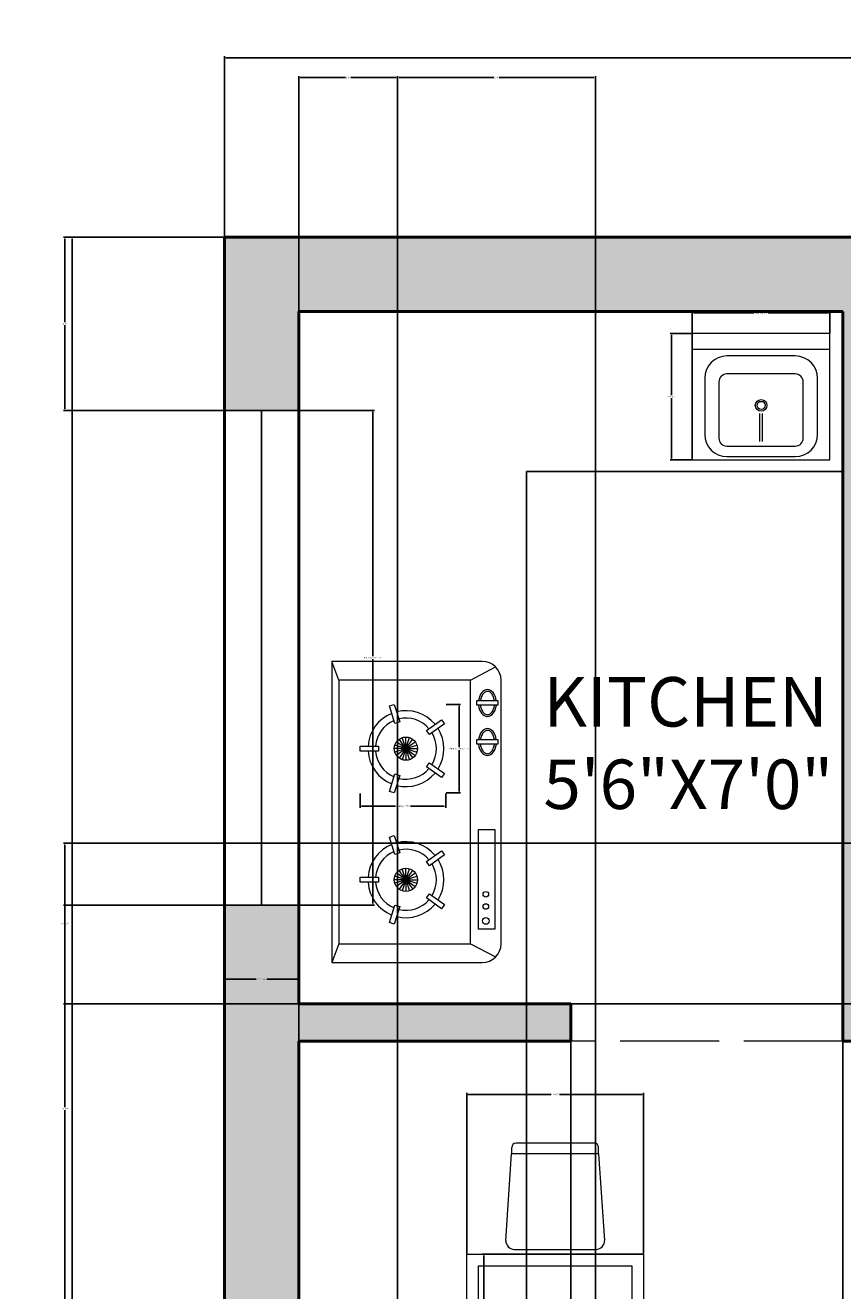
# Model space of a CAD drawing. Units: inches. Extents: x -2 to 282, y -370 to 35.
# Tile 4 of 5: x -2 to 97, y -119 to 35. Entities that reach past the tile are written whole.
import ezdxf

# ---------------------------------------------------------------- set-up
doc = ezdxf.new("R2010")
doc.units = ezdxf.units.IN
doc.header["$MEASUREMENT"] = 0
doc.linetypes.add('ACAD_ISO02W100', pattern=[15, 12, -3])
for name, color, linetype, lineweight in [('A-ANNO-DIMS', 2, 'Continuous', 18), ('A-AREA-IDEN', 7, 'Continuous', 25), ('A-EQPM', 8, 'Continuous', 18), ('A-FLOR-CASE', 8, 'Continuous', 25), ('A-FLOR-FIXT', 9, 'Continuous', 18), ('A-FURN', 8, 'Continuous', 18), ('A-GLAZ', 4, 'Continuous', 25), ('A-WALL', 7, 'Continuous', 50), ('A-WALL-OVHD', 7, 'ACAD_ISO02W100', 18), ('A-WALL-PATT', 252, 'Continuous', 13)]:
    doc.layers.add(name, color=color, linetype=linetype, lineweight=lineweight)
doc.styles.get("Standard").update_dxf_attribs({"font": 'arial.ttf'})
doc.dimstyles.get("Standard").update_dxf_attribs({"dimtxt": 0.18, "dimasz": 0.18, "dimexe": 0.18, "dimexo": 0.0625, "dimgap": 0.09, "dimtad": 0, "dimtih": 1, "dimtoh": 1, "dimdec": 0, "dimzin": 0, "dimdsep": 46, "dimlunit": 3, "dimtxsty": 'Standard', "dimcen": 0.09, "dimadec": 0, "dimazin": 0, "dimtfac": 1, "dimtdec": 0, "dimtofl": 0, "dimtmove": 0, "dimatfit": 3, "dimfxl": 1, "dimtolj": 1, "dimtzin": 0, "dimarcsym": 0})

# ---------------------------------------------------------------- blocks, each defined once
blk = doc.blocks.new('*D2')
at = {"layer": 'A-ANNO-DIMS', "color": 0, "lineweight": -2, "transparency": 16777216}
for p, q in [((22.35, 9.19), (3.74, 9.19)), ((3.92, 9.01), (3.92, -167.65)), ((3.92, -350.63), (3.92, -173.97)), ((22.35, -350.81), (3.74, -350.81))]:
    blk.add_line(p, q, dxfattribs=at)
at = {"layer": 'A-ANNO-DIMS', "color": 0, "transparency": 16777216}
for points in [[(3.89, 9.01), (3.95, 9.01), (3.92, 9.19)], [(3.89, -350.63), (3.95, -350.63), (3.92, -350.81)]]:
    blk.add_solid(points, dxfattribs=at)
at = {"layer": 'Defpoints', "color": 0, "transparency": 16777216}
for p in [(3.92, 9.19), (22.41, 9.19), (22.41, -350.81)]:
    blk.add_point(p, dxfattribs=at)
at = {"layer": 'A-ANNO-DIMS', "color": 0, "transparency": 16777216, "insert": (3.92, -170.81), "char_height": 6, "attachment_point": 5}
blk.add_mtext("\\A1;30'", dxfattribs=at)
blk = doc.blocks.new('*D3')
at = {"layer": 'A-ANNO-DIMS', "color": 0, "lineweight": -2, "transparency": 16777216}
for p, q in [((22.41, 9.25), (22.41, 31.14)), ((22.59, 30.96), (137.18, 30.96)), ((262.23, 30.96), (147.65, 30.96)), ((262.41, 9.25), (262.41, 31.14))]:
    blk.add_line(p, q, dxfattribs=at)
at = {"layer": 'A-ANNO-DIMS', "color": 0, "transparency": 16777216}
for points in [[(22.59, 30.99), (22.59, 30.93), (22.41, 30.96)], [(262.23, 30.99), (262.23, 30.93), (262.41, 30.96)]]:
    blk.add_solid(points, dxfattribs=at)
at = {"layer": 'Defpoints', "color": 0, "transparency": 16777216}
for p in [(262.41, 30.96), (22.41, 9.19), (262.41, 9.19)]:
    blk.add_point(p, dxfattribs=at)
at = {"layer": 'A-ANNO-DIMS', "color": 0, "transparency": 16777216, "insert": (142.41, 30.96), "char_height": 6, "attachment_point": 5}
blk.add_mtext("\\A1;20'", dxfattribs=at)
blk = doc.blocks.new('М14 600х655')
for p, q in [((-655, 600), (-655, 0)), ((-655, 600), (-655, 0)), ((-655, 0), (-655, 600)), ((0, 600), (-655, 600)), ((0, 0), (0, 600)), ((0, 525), (-655, 525)), ((-165.1, 494.1), (-489.9, 494.1)), ((-595.8, 388.1), (-595.8, 121.3)), ((-528.4, 370.1), (-528.4, 103.3)), ((-165.4, 408.4), (-490.2, 408.4)), ((-127.2, 103.3), (-127.2, 370.1)), ((-59.2, 121.3), (-59.2, 388.1)), ((-333.5, 87.1), (-333.5, 219.6)), ((-321.5, 87.1), (-321.5, 219.6)), ((-490.2, 65.1), (-165.4, 65.1)), ((-655, 0), (-655, 0)), ((-655, 0), (-655, 0)), ((-655, 0), (0, 0)), ((-655, 0), (0, 0)), ((-489.9, 15.4), (-165.1, 15.4))]:
    blk.add_line(p, q)
for radius in [27.6, 19.3]:
    blk.add_circle((-327.5, 258.9), radius)
for centre, radius, start, end in [((-489.9, 388.1), 105.9, 90, 180), ((-165.1, 388.1), 105.9, 0, 90), ((-490.2, 370.1), 38.2, 90, 180), ((-165.4, 370.1), 38.2, 0, 90), ((-489.9, 121.3), 105.9, 180, 270), ((-165.1, 121.3), 105.9, 270, 0), ((-490.2, 103.3), 38.2, 180, 270), ((-165.4, 103.3), 38.2, 270, 0)]:
    blk.add_arc(centre, radius, start, end)
blk = doc.blocks.new('WINDOW-60IN')
for p, q in [((0, 0), (0, 60)), ((0, 60), (9, 60)), ((4.5, 60), (4.5, 0)), ((9, 60), (9, 0)), ((9, 0), (0, 0))]:
    blk.add_line(p, q)
blk = doc.blocks.new('DINING-CHAIR')
for p, q in [((0.71, 12.36), (0.71, 11.58)), ((10.75, 12.87), (1.23, 12.87)), ((11.26, 11.58), (11.26, 12.36)), ((0, 1.09), (0.71, 11.58)), ((11.26, 11.58), (0.71, 11.58)), ((11.26, 11.58), (11.98, 1.09)), ((1.03, 0), (10.95, 0))]:
    blk.add_line(p, q)
for centre, radius, start, end in [((1.23, 12.36), 0.515, 90, 180), ((10.75, 12.36), 0.515, 0, 90), ((1.03, 1.03), 1.03, 176.8779, 270), ((10.95, 1.03), 1.03, 270, 3.1221)]:
    blk.add_arc(centre, radius, start, end)
blk = doc.blocks.new('COOKTOP-BURNER')
for p, q in [((3.54, 10.55), (4.13, 10.74)), ((4.22, 8.44), (3.54, 10.55)), ((4.13, 10.74), (4.82, 8.63)), ((4.82, 8.63), (4.22, 8.44)), ((8.06, 7.58), (9.85, 8.88)), ((10.22, 8.38), (8.42, 7.07)), ((9.85, 8.88), (10.22, 8.38)), ((5.55, 5.37), (4.41, 6.2)), ((5.55, 5.37), (4.72, 6.51)), ((5.55, 5.37), (5.11, 6.71)), ((5.55, 5.37), (5.55, 6.78)), ((5.55, 5.37), (5.98, 6.71)), ((5.55, 5.37), (6.37, 6.51)), ((5.55, 5.37), (6.69, 6.2)), ((8.42, 7.07), (8.06, 7.58)), ((0, 5.06), (0, 5.68)), ((0, 5.68), (2.22, 5.68)), ((2.22, 5.06), (0, 5.06)), ((2.22, 5.68), (2.22, 5.06)), ((5.55, 5.37), (4.14, 5.37)), ((5.55, 5.37), (4.21, 5.81)), ((5.55, 5.37), (4.21, 4.94)), ((5.55, 5.37), (4.41, 4.54)), ((5.55, 5.37), (4.72, 4.23)), ((5.55, 5.37), (5.11, 4.03)), ((5.55, 5.37), (6.89, 5.81)), ((5.55, 5.37), (6.95, 5.37)), ((5.55, 5.37), (6.89, 4.94)), ((5.55, 5.37), (6.69, 4.54)), ((5.55, 5.37), (6.37, 4.23)), ((5.55, 5.37), (5.98, 4.03)), ((5.55, 5.37), (5.55, 3.96)), ((8.06, 3.16), (8.42, 3.67)), ((9.85, 1.86), (8.06, 3.16)), ((8.42, 3.67), (10.22, 2.36)), ((3.54, 0.19), (4.22, 2.3)), ((4.82, 2.11), (4.13, 0)), ((4.22, 2.3), (4.82, 2.11)), ((10.22, 2.36), (9.85, 1.86)), ((4.13, 0), (3.54, 0.19))]:
    blk.add_line(p, q)
blk.add_circle((5.55, 5.37), 1.41)
for radius, start, end in [(4.61, 111.8765, 176.1235), (4.61, 39.8765, 104.1235), (3.7, 112.8365, 175.1635), (3.7, 40.8365, 103.1635), (4.61, 327.8765, 32.1235), (3.7, 328.8365, 31.1635), (4.61, 183.8765, 248.1235), (3.7, 184.8365, 247.1635), (4.61, 255.8765, 320.1235), (3.7, 256.8365, 319.1635)]:
    blk.add_arc((5.55, 5.37), radius, start, end)
blk = doc.blocks.new('*D11')
at = {"layer": 'A-ANNO-DIMS', "color": 0, "lineweight": -2, "transparency": 16777216}
for p, q in [((31.48, -11.81), (40.59, -11.81)), ((40.41, -11.99), (40.41, -41.63)), ((40.41, -71.63), (40.41, -41.99)), ((31.48, -71.81), (40.59, -71.81))]:
    blk.add_line(p, q, dxfattribs=at)
at = {"layer": 'A-ANNO-DIMS', "color": 0, "transparency": 16777216}
for points in [[(40.38, -11.99), (40.44, -11.99), (40.41, -11.81)], [(40.38, -71.63), (40.44, -71.63), (40.41, -71.81)]]:
    blk.add_solid(points, dxfattribs=at)
at = {"layer": 'Defpoints', "color": 0, "transparency": 16777216}
for p in [(31.41, -11.81), (40.41, -11.81), (31.41, -71.81)]:
    blk.add_point(p, dxfattribs=at)
at = {"layer": 'A-ANNO-DIMS', "color": 0, "transparency": 16777216, "insert": (40.41, -41.81), "char_height": 0.18, "attachment_point": 5}
blk.add_mtext('\\A1;WINDOW 5\'-0" TYP.', dxfattribs=at)
blk = doc.blocks.new('*D12')
at = {"layer": 'A-ANNO-DIMS', "color": 0, "lineweight": -2, "transparency": 16777216}
for p, q in [((22.41, -71.87), (22.41, -80.99)), ((31.41, -71.87), (31.41, -80.99)), ((22.59, -80.81), (26.27, -80.81)), ((31.23, -80.81), (27.55, -80.81))]:
    blk.add_line(p, q, dxfattribs=at)
at = {"layer": 'A-ANNO-DIMS', "color": 0, "transparency": 16777216}
for points in [[(22.59, -80.78), (22.59, -80.84), (22.41, -80.81)], [(31.23, -80.78), (31.23, -80.84), (31.41, -80.81)]]:
    blk.add_solid(points, dxfattribs=at)
at = {"layer": 'Defpoints', "color": 0, "transparency": 16777216}
for p in [(22.41, -71.81), (31.41, -71.81), (31.41, -80.81)]:
    blk.add_point(p, dxfattribs=at)
at = {"layer": 'A-ANNO-DIMS', "color": 0, "transparency": 16777216, "insert": (26.91, -80.81), "char_height": 0.18, "attachment_point": 5}
blk.add_mtext('\\A1;0\'-9" TYP.', dxfattribs=at)
blk = doc.blocks.new('*D21')
at = {"layer": 'A-ANNO-DIMS', "color": 0, "lineweight": -2, "transparency": 16777216}
for p, q in [((49.32, -47.47), (51.05, -47.47)), ((50.87, -47.65), (50.87, -52.66)), ((50.87, -58.03), (50.87, -53.02)), ((49.32, -58.21), (51.05, -58.21))]:
    blk.add_line(p, q, dxfattribs=at)
at = {"layer": 'A-ANNO-DIMS', "color": 0, "transparency": 16777216}
for points in [[(50.84, -47.65), (50.9, -47.65), (50.87, -47.47)], [(50.84, -58.03), (50.9, -58.03), (50.87, -58.21)]]:
    blk.add_solid(points, dxfattribs=at)
at = {"layer": 'Defpoints', "color": 0, "transparency": 16777216}
for p in [(49.26, -47.47), (50.87, -47.47), (49.26, -58.21)]:
    blk.add_point(p, dxfattribs=at)
at = {"layer": 'A-ANNO-DIMS', "color": 0, "transparency": 16777216, "insert": (50.87, -52.84), "char_height": 0.18, "attachment_point": 5}
blk.add_mtext('\\A1;BURNER 0\'-10 1/2" TYP.', dxfattribs=at)
blk = doc.blocks.new('*D22')
at = {"layer": 'A-ANNO-DIMS', "color": 0, "lineweight": -2, "transparency": 16777216}
for p, q in [((38.87, -58.27), (38.87, -60)), ((49.26, -58.27), (49.26, -60)), ((39.05, -59.82), (43.15, -59.82)), ((49.08, -59.82), (44.99, -59.82))]:
    blk.add_line(p, q, dxfattribs=at)
at = {"layer": 'A-ANNO-DIMS', "color": 0, "transparency": 16777216}
for points in [[(39.05, -59.79), (39.05, -59.85), (38.87, -59.82)], [(49.08, -59.79), (49.08, -59.85), (49.26, -59.82)]]:
    blk.add_solid(points, dxfattribs=at)
at = {"layer": 'Defpoints', "color": 0, "transparency": 16777216}
for p in [(38.87, -58.21), (49.26, -58.21), (49.26, -59.82)]:
    blk.add_point(p, dxfattribs=at)
at = {"layer": 'A-ANNO-DIMS', "color": 0, "transparency": 16777216, "insert": (44.07, -59.82), "char_height": 0.18, "attachment_point": 5}
blk.add_mtext('\\A1;0\'-10 1/2" TYP.', dxfattribs=at)
blk = doc.blocks.new('*D23')
at = {"layer": 'A-ANNO-DIMS', "color": 0, "lineweight": -2, "transparency": 16777216}
for p, q in [((79.16, -2.44), (79.16, 0.19)), ((79.34, 0.01), (86.64, 0.01)), ((95.69, 0.01), (88.38, 0.01)), ((95.87, -2.44), (95.87, 0.19))]:
    blk.add_line(p, q, dxfattribs=at)
at = {"layer": 'A-ANNO-DIMS', "color": 0, "transparency": 16777216}
for points in [[(79.34, 0.04), (79.34, -0.02), (79.16, 0.01)], [(95.69, 0.04), (95.69, -0.02), (95.87, 0.01)]]:
    blk.add_solid(points, dxfattribs=at)
at = {"layer": 'Defpoints', "color": 0, "transparency": 16777216}
for p in [(95.87, 0.01), (79.16, -2.5), (95.87, -2.5)]:
    blk.add_point(p, dxfattribs=at)
at = {"layer": 'A-ANNO-DIMS', "color": 0, "transparency": 16777216, "insert": (87.51, 0.01), "char_height": 0.18, "attachment_point": 5}
blk.add_mtext('\\A1;SINK 1\'-4 1/2"', dxfattribs=at)
blk = doc.blocks.new('*D24')
at = {"layer": 'A-ANNO-DIMS', "color": 0, "lineweight": -2, "transparency": 16777216}
for p, q in [((79.09, -2.5), (76.47, -2.5)), ((76.65, -2.68), (76.65, -9.97)), ((76.65, -17.63), (76.65, -10.34)), ((79.09, -17.81), (76.47, -17.81))]:
    blk.add_line(p, q, dxfattribs=at)
at = {"layer": 'A-ANNO-DIMS', "color": 0, "transparency": 16777216}
for points in [[(76.62, -2.68), (76.68, -2.68), (76.65, -2.5)], [(76.62, -17.63), (76.68, -17.63), (76.65, -17.81)]]:
    blk.add_solid(points, dxfattribs=at)
at = {"layer": 'Defpoints', "color": 0, "transparency": 16777216}
for p in [(76.65, -2.5), (79.16, -2.5), (79.16, -17.81)]:
    blk.add_point(p, dxfattribs=at)
at = {"layer": 'A-ANNO-DIMS', "color": 0, "transparency": 16777216, "insert": (76.65, -10.15), "char_height": 0.18, "attachment_point": 5}
blk.add_mtext('\\A1;1\'-3 1/2"', dxfattribs=at)
blk = doc.blocks.new('*D29')
at = {"layer": 'A-ANNO-DIMS', "color": 0, "lineweight": -2, "transparency": 16777216}
for p, q in [((22.35, 9.19), (2.86, 9.19)), ((3.04, 9.01), (3.04, -1.13)), ((3.04, -11.63), (3.04, -1.49)), ((22.35, -11.81), (2.86, -11.81))]:
    blk.add_line(p, q, dxfattribs=at)
at = {"layer": 'A-ANNO-DIMS', "color": 0, "transparency": 16777216}
for points in [[(3.01, 9.01), (3.07, 9.01), (3.04, 9.19)], [(3.01, -11.63), (3.07, -11.63), (3.04, -11.81)]]:
    blk.add_solid(points, dxfattribs=at)
at = {"layer": 'Defpoints', "color": 0, "transparency": 16777216}
for p in [(22.41, 9.19), (3.04, -11.81), (22.41, -11.81)]:
    blk.add_point(p, dxfattribs=at)
at = {"layer": 'A-ANNO-DIMS', "color": 0, "transparency": 16777216, "insert": (3.04, -1.31), "char_height": 0.18, "attachment_point": 5}
blk.add_mtext('\\A1;1\'-9"', dxfattribs=at)
blk = doc.blocks.new('*D30')
at = {"layer": 'A-ANNO-DIMS', "color": 0, "lineweight": -2, "transparency": 16777216}
for p, q in [((22.35, -71.81), (2.86, -71.81)), ((3.04, -71.99), (3.04, -96.32)), ((3.04, -121.02), (3.04, -96.69)), ((22.35, -121.2), (2.86, -121.2))]:
    blk.add_line(p, q, dxfattribs=at)
at = {"layer": 'A-ANNO-DIMS', "color": 0, "transparency": 16777216}
for points in [[(3.01, -71.99), (3.07, -71.99), (3.04, -71.81)], [(3.01, -121.02), (3.07, -121.02), (3.04, -121.2)]]:
    blk.add_solid(points, dxfattribs=at)
at = {"layer": 'Defpoints', "color": 0, "transparency": 16777216}
for p in [(22.41, -71.81), (3.04, -121.2), (22.41, -121.2)]:
    blk.add_point(p, dxfattribs=at)
at = {"layer": 'A-ANNO-DIMS', "color": 0, "transparency": 16777216, "insert": (3.04, -96.51), "char_height": 0.18, "attachment_point": 5}
blk.add_mtext('\\A1;4\'-1 1/2"', dxfattribs=at)
blk = doc.blocks.new('*D37')
at = {"layer": 'A-ANNO-DIMS', "color": 0, "lineweight": -2, "transparency": 16777216}
for p, q in [((31.41, -277.25), (31.41, 28.74)), ((31.59, 28.56), (37.09, 28.56)), ((43.23, 28.56), (37.73, 28.56)), ((43.41, -277.25), (43.41, 28.74))]:
    blk.add_line(p, q, dxfattribs=at)
at = {"layer": 'A-ANNO-DIMS', "color": 0, "transparency": 16777216}
for points in [[(31.59, 28.59), (31.59, 28.53), (31.41, 28.56)], [(43.23, 28.59), (43.23, 28.53), (43.41, 28.56)]]:
    blk.add_solid(points, dxfattribs=at)
at = {"layer": 'Defpoints', "color": 0, "transparency": 16777216}
for p in [(43.41, 28.56), (31.41, -277.31), (43.41, -277.31)]:
    blk.add_point(p, dxfattribs=at)
at = {"layer": 'A-ANNO-DIMS', "color": 0, "transparency": 16777216, "insert": (37.41, 28.56), "char_height": 0.18, "attachment_point": 5}
blk.add_mtext('\\A1;1\'-0"', dxfattribs=at)
blk = doc.blocks.new('*D38')
at = {"layer": 'A-ANNO-DIMS', "color": 0, "lineweight": -2, "transparency": 16777216}
for p, q in [((43.41, -277.25), (43.41, 28.74)), ((43.59, 28.56), (55.08, 28.56)), ((67.23, 28.56), (55.74, 28.56)), ((67.41, -277.25), (67.41, 28.74))]:
    blk.add_line(p, q, dxfattribs=at)
at = {"layer": 'A-ANNO-DIMS', "color": 0, "transparency": 16777216}
for points in [[(43.59, 28.59), (43.59, 28.53), (43.41, 28.56)], [(67.23, 28.59), (67.23, 28.53), (67.41, 28.56)]]:
    blk.add_solid(points, dxfattribs=at)
at = {"layer": 'Defpoints', "color": 0, "transparency": 16777216}
for p in [(67.41, 28.56), (43.41, -277.31), (67.41, -277.31)]:
    blk.add_point(p, dxfattribs=at)
at = {"layer": 'A-ANNO-DIMS', "color": 0, "transparency": 16777216, "insert": (55.41, 28.56), "char_height": 0.18, "attachment_point": 5}
blk.add_mtext('\\A1;2\'-0"', dxfattribs=at)
blk = doc.blocks.new('*D39')
at = {"layer": 'A-ANNO-DIMS', "color": 0, "lineweight": -2, "transparency": 16777216}
for p, q in [((64.41, -88.37), (64.41, -370.37)), ((97.41, -88.37), (97.41, -370.37)), ((64.59, -370.19), (80.58, -370.19)), ((97.23, -370.19), (81.24, -370.19))]:
    blk.add_line(p, q, dxfattribs=at)
at = {"layer": 'A-ANNO-DIMS', "color": 0, "transparency": 16777216}
for points in [[(64.59, -370.16), (64.59, -370.22), (64.41, -370.19)], [(97.23, -370.16), (97.23, -370.22), (97.41, -370.19)]]:
    blk.add_solid(points, dxfattribs=at)
at = {"layer": 'Defpoints', "color": 0, "transparency": 16777216}
for p in [(64.41, -88.31), (97.41, -88.31), (97.41, -370.19)]:
    blk.add_point(p, dxfattribs=at)
at = {"layer": 'A-ANNO-DIMS', "color": 0, "transparency": 16777216, "insert": (80.91, -370.19), "char_height": 0.18, "attachment_point": 5}
blk.add_mtext('\\A1;2\'-9"', dxfattribs=at)
blk = doc.blocks.new('*D42')
at = {"layer": 'A-ANNO-DIMS', "color": 0, "lineweight": -2, "transparency": 16777216}
for p, q in [((31.41, -83.87), (31.41, -370.37)), ((59.05, -83.87), (59.05, -370.37)), ((31.59, -370.19), (44.69, -370.19)), ((58.87, -370.19), (45.77, -370.19))]:
    blk.add_line(p, q, dxfattribs=at)
at = {"layer": 'A-ANNO-DIMS', "color": 0, "transparency": 16777216}
for points in [[(31.59, -370.16), (31.59, -370.22), (31.41, -370.19)], [(58.87, -370.16), (58.87, -370.22), (59.05, -370.19)]]:
    blk.add_solid(points, dxfattribs=at)
at = {"layer": 'Defpoints', "color": 0, "transparency": 16777216}
for p in [(31.41, -83.81), (59.05, -83.81), (59.05, -370.19)]:
    blk.add_point(p, dxfattribs=at)
at = {"layer": 'A-ANNO-DIMS', "color": 0, "transparency": 16777216, "insert": (45.23, -370.19), "char_height": 0.18, "attachment_point": 5}
blk.add_mtext('\\A1;2\'-3 1/2"', dxfattribs=at)
blk = doc.blocks.new('*D45')
at = {"layer": 'A-ANNO-DIMS', "color": 0, "lineweight": -2, "transparency": 16777216}
for p, q in [((101.85, -64.31), (2.86, -64.31)), ((3.04, -64.49), (3.04, -73.88)), ((3.04, -83.63), (3.04, -74.24)), ((101.85, -83.81), (2.86, -83.81))]:
    blk.add_line(p, q, dxfattribs=at)
at = {"layer": 'A-ANNO-DIMS', "color": 0, "transparency": 16777216}
for points in [[(3.01, -64.49), (3.07, -64.49), (3.04, -64.31)], [(3.01, -83.63), (3.07, -83.63), (3.04, -83.81)]]:
    blk.add_solid(points, dxfattribs=at)
at = {"layer": 'Defpoints', "color": 0, "transparency": 16777216}
for p in [(101.91, -64.31), (3.04, -83.81), (101.91, -83.81)]:
    blk.add_point(p, dxfattribs=at)
at = {"layer": 'A-ANNO-DIMS', "color": 0, "transparency": 16777216, "insert": (3.04, -74.06), "char_height": 0.18, "attachment_point": 5}
blk.add_mtext('\\A1;1\'-7 1/2"', dxfattribs=at)
blk = doc.blocks.new('*D50')
at = {"layer": 'A-ANNO-DIMS', "color": 0, "lineweight": -2, "transparency": 16777216}
for p, q in [((73.19, -114.14), (53.7, -114.14)), ((53.88, -114.32), (53.88, -124.68)), ((53.88, -135.41), (53.88, -125.05)), ((73.19, -135.59), (53.7, -135.59))]:
    blk.add_line(p, q, dxfattribs=at)
at = {"layer": 'A-ANNO-DIMS', "color": 0, "transparency": 16777216}
for points in [[(53.85, -114.32), (53.91, -114.32), (53.88, -114.14)], [(53.85, -135.41), (53.91, -135.41), (53.88, -135.59)]]:
    blk.add_solid(points, dxfattribs=at)
at = {"layer": 'Defpoints', "color": 0, "transparency": 16777216}
for p in [(53.88, -114.14), (73.25, -114.14), (73.25, -135.59)]:
    blk.add_point(p, dxfattribs=at)
at = {"layer": 'A-ANNO-DIMS', "color": 0, "transparency": 16777216, "insert": (53.88, -124.87), "char_height": 0.18, "attachment_point": 5}
blk.add_mtext('\\A1;1\'-9 1/2"', dxfattribs=at)
blk = doc.blocks.new('*D51')
at = {"layer": 'A-ANNO-DIMS', "color": 0, "lineweight": -2, "transparency": 16777216}
for p, q in [((51.8, -114.08), (51.8, -94.59)), ((51.98, -94.77), (62, -94.77)), ((73.07, -94.77), (63.06, -94.77)), ((73.25, -114.08), (73.25, -94.59))]:
    blk.add_line(p, q, dxfattribs=at)
at = {"layer": 'A-ANNO-DIMS', "color": 0, "transparency": 16777216}
for points in [[(51.98, -94.74), (51.98, -94.8), (51.8, -94.77)], [(73.07, -94.74), (73.07, -94.8), (73.25, -94.77)]]:
    blk.add_solid(points, dxfattribs=at)
at = {"layer": 'Defpoints', "color": 0, "transparency": 16777216}
for p in [(73.25, -94.77), (51.8, -114.14), (73.25, -114.14)]:
    blk.add_point(p, dxfattribs=at)
at = {"layer": 'A-ANNO-DIMS', "color": 0, "transparency": 16777216, "insert": (62.53, -94.77), "char_height": 0.18, "attachment_point": 5}
blk.add_mtext('\\A1;1\'-9 1/2"', dxfattribs=at)

msp = doc.modelspace()

# ---------------------------------------------------------------- hatches: boundary and pattern name
at = {"layer": 'A-WALL-PATT'}
h = msp.add_hatch(color=256, dxfattribs=at)
h.dxf.hatch_style = 1
h.paths.add_polyline_path([(262.41, 9.19), (134.91, 9.19), (134.91, 0.19), (143.91, 0.19), (143.91, -35.81), (148.41, -35.81), (148.41, 0.19), (253.41, 0.19), (253.41, -29.06), (262.41, -29.06)])
h.paths.add_polyline_path([(110.91, 9.19), (22.41, 9.19), (22.41, -11.81), (31.41, -11.81), (31.41, 0.19), (97.41, 0.19), (97.41, -88.31), (101.91, -88.31), (101.91, -64.31), (143.91, -64.31), (143.91, -88.31), (148.41, -88.31), (148.41, -59.81), (101.91, -59.81), (101.91, 0.19), (110.91, 0.19)])
h.paths.add_polyline_path([(31.41, -88.31), (64.41, -88.31), (64.41, -83.81), (31.41, -83.81), (31.41, -71.81), (22.41, -71.81), (22.41, -121.2), (31.41, -121.2)])
h.paths.add_polyline_path([(262.41, -89.06), (253.41, -89.06), (253.41, -118.31), (143.91, -118.31), (143.91, -122.81), (184.41, -122.81), (184.41, -164.81), (184.41, -169.31), (188.91, -169.31), (188.91, -164.81), (188.91, -122.81), (253.41, -122.81), (253.41, -131.81), (262.41, -131.81)])
h.paths.add_polyline_path([(262.41, -155.81), (253.41, -155.81), (253.41, -164.81), (212.91, -164.81), (212.91, -169.31), (253.41, -169.31), (253.41, -193.31), (262.41, -193.31)])
h.paths.add_polyline_path([(262.41, -253.31), (253.41, -253.31), (253.41, -277.31), (148.41, -277.31), (148.41, -164.81), (143.91, -164.81), (143.91, -169.31), (143.91, -281.81), (253.41, -281.81), (253.41, -341.81), (143.91, -341.81), (143.91, -350.81), (262.41, -350.81)])
h.paths.add_polyline_path([(31.41, -323.81), (22.41, -323.81), (22.41, -350.81), (95.91, -350.81), (95.91, -281.81), (107.91, -281.81), (107.91, -277.31), (67.41, -277.31), (67.41, -281.81), (91.41, -281.81), (91.41, -341.81), (31.41, -341.81)])
h.paths.add_polyline_path([(43.41, -277.31), (31.41, -277.31), (31.41, -181.2), (22.41, -181.2), (22.41, -299.81), (31.41, -299.81), (31.41, -281.81), (43.41, -281.81)])

# ---------------------------------------------------------------- linework, layer by layer
at = {"layer": 'A-EQPM'}
for p, q in [((53.69, -42.25), (35.43, -42.25)), ((35.43, -42.25), (35.43, -78.78)), ((36.29, -44.54), (35.43, -42.25)), ((52.27, -44.54), (55.3, -42.92)), ((52.27, -44.54), (36.29, -44.54)), ((36.29, -44.54), (36.29, -76.5)), ((52.27, -76.5), (52.27, -44.54)), ((55.97, -76.5), (55.97, -44.54)), ((53.03, -47.57), (53.03, -46.98)), ((53.03, -46.98), (55.56, -46.98)), ((55.56, -47.57), (53.03, -47.57)), ((55.56, -46.98), (55.56, -47.57)), ((53.03, -51.71), (55.56, -51.71)), ((53.03, -52.3), (53.03, -51.71)), ((55.56, -51.71), (55.56, -52.3)), ((55.56, -52.3), (53.03, -52.3)), ((53.23, -74.75), (53.23, -62.66)), ((53.23, -62.66), (55.19, -62.66)), ((55.19, -62.66), (55.19, -74.75)), ((55.19, -74.75), (53.23, -74.75)), ((36.29, -76.5), (35.43, -78.78)), ((36.29, -76.5), (52.27, -76.5)), ((52.27, -76.5), (55.3, -78.11)), ((35.43, -78.78), (53.69, -78.78))]:
    msp.add_line(p, q, dxfattribs=at)
for centre, radius in [((54.11, -70.5), 0.337), ((54.11, -71.98), 0.337), ((54.11, -73.74), 0.405)]:
    msp.add_circle(centre, radius, dxfattribs=at)
for centre, start, end in [((53.69, -44.54), 0, 90), ((53.69, -76.5), 270, 0)]:
    msp.add_arc(centre, 2.28, start, end, dxfattribs=at)
for centre, major_axis, start_param, end_param in [((54.31, -47.31), (0, -1.63), 1.774361, 4.508825), ((54.31, -47.31), (0, 1.63), 1.73081, 4.552375), ((54.31, -52.04), (0, -1.63), 1.774361, 4.508825), ((54.31, -52.04), (0, 1.63), 1.73081, 4.552375)]:
    msp.add_ellipse(centre, major_axis=major_axis, ratio=0.671641, start_param=start_param, end_param=end_param, dxfattribs=at)
for points, knots in [([(55.15, -46.98), (55.14, -46.9), (55.12, -46.82), (55.08, -46.65), (55.04, -46.56), (54.96, -46.39), (54.92, -46.31), (54.82, -46.18), (54.76, -46.12), (54.66, -46.02), (54.6, -45.99), (54.49, -45.93), (54.43, -45.92), (54.32, -45.9), (54.27, -45.91), (54.16, -45.93), (54.1, -45.95), (53.99, -46.01), (53.93, -46.05), (53.82, -46.15), (53.77, -46.21), (53.68, -46.35), (53.63, -46.43), (53.56, -46.61), (53.52, -46.7), (53.49, -46.86), (53.47, -46.92), (53.46, -46.98)], [8.079302, 8.079302, 8.079302, 8.079302, 8.245651, 8.245651, 8.463703, 8.463703, 8.681755, 8.681755, 8.899807, 8.899807, 9.117859, 9.117859, 9.33591, 9.33591, 9.553962, 9.553962, 9.772014, 9.772014, 9.990066, 9.990066, 10.208118, 10.208118, 10.426169, 10.426169, 10.644221, 10.644221, 10.770253, 10.770253, 10.770253, 10.770253]), ([(53.46, -47.57), (53.46, -47.63), (53.47, -47.69), (53.51, -47.85), (53.54, -47.95), (53.61, -48.13), (53.65, -48.22), (53.74, -48.37), (53.79, -48.43), (53.9, -48.55), (53.95, -48.59), (54.06, -48.66), (54.12, -48.69), (54.22, -48.71), (54.26, -48.72), (54.31, -48.72), (54.36, -48.72), (54.42, -48.71), (54.53, -48.67), (54.59, -48.64), (54.7, -48.57), (54.75, -48.52), (54.86, -48.4), (54.91, -48.33), (54.99, -48.17), (55.03, -48.09), (55.1, -47.9), (55.13, -47.8), (55.15, -47.66), (55.16, -47.61), (55.16, -47.57)], [4.889299, 4.889299, 4.889299, 4.889299, 5.015191, 5.015191, 5.233243, 5.233243, 5.451295, 5.451295, 5.669347, 5.669347, 5.887399, 5.887399, 6.10545, 6.10545, 6.283185, 6.283185, 6.283185, 6.501237, 6.501237, 6.719289, 6.719289, 6.937341, 6.937341, 7.155392, 7.155392, 7.373444, 7.373444, 7.591496, 7.591496, 7.677072, 7.677072, 7.677072, 7.677072]), ([(55.15, -51.71), (55.14, -51.63), (55.12, -51.55), (55.08, -51.38), (55.04, -51.29), (54.96, -51.12), (54.92, -51.04), (54.82, -50.91), (54.76, -50.85), (54.66, -50.75), (54.6, -50.72), (54.49, -50.66), (54.43, -50.65), (54.32, -50.63), (54.27, -50.63), (54.16, -50.66), (54.1, -50.68), (53.99, -50.74), (53.93, -50.78), (53.82, -50.88), (53.77, -50.94), (53.68, -51.08), (53.63, -51.16), (53.56, -51.34), (53.52, -51.43), (53.49, -51.59), (53.47, -51.65), (53.46, -51.71)], [8.079302, 8.079302, 8.079302, 8.079302, 8.245651, 8.245651, 8.463703, 8.463703, 8.681755, 8.681755, 8.899807, 8.899807, 9.117859, 9.117859, 9.33591, 9.33591, 9.553962, 9.553962, 9.772014, 9.772014, 9.990066, 9.990066, 10.208118, 10.208118, 10.426169, 10.426169, 10.644221, 10.644221, 10.770253, 10.770253, 10.770253, 10.770253]), ([(53.46, -52.3), (53.46, -52.36), (53.47, -52.42), (53.51, -52.58), (53.54, -52.68), (53.61, -52.86), (53.65, -52.95), (53.74, -53.1), (53.79, -53.16), (53.9, -53.28), (53.95, -53.32), (54.06, -53.39), (54.12, -53.41), (54.22, -53.44), (54.26, -53.45), (54.31, -53.45), (54.36, -53.45), (54.42, -53.44), (54.53, -53.4), (54.59, -53.37), (54.7, -53.3), (54.75, -53.25), (54.86, -53.13), (54.91, -53.06), (54.99, -52.9), (55.03, -52.81), (55.1, -52.63), (55.13, -52.53), (55.15, -52.38), (55.16, -52.34), (55.16, -52.3)], [4.889299, 4.889299, 4.889299, 4.889299, 5.015191, 5.015191, 5.233243, 5.233243, 5.451295, 5.451295, 5.669347, 5.669347, 5.887399, 5.887399, 6.10545, 6.10545, 6.283185, 6.283185, 6.283185, 6.501237, 6.501237, 6.719289, 6.719289, 6.937341, 6.937341, 7.155392, 7.155392, 7.373444, 7.373444, 7.591496, 7.591496, 7.677072, 7.677072, 7.677072, 7.677072])]:
    msp.add_open_spline(points, degree=3, knots=knots, dxfattribs=at)
at = {"layer": 'A-FLOR-CASE'}
for p, q in [((59.05, -83.81), (59.05, -19.21)), ((59.05, -19.21), (97.41, -19.21))]:
    msp.add_line(p, q, dxfattribs=at)
at = {"layer": 'A-FURN'}
for points in [[(51.8, -135.59), (51.8, -114.14), (73.25, -114.14), (73.25, -135.59)], [(53.23, -134.16), (53.23, -115.57), (71.82, -115.57), (71.82, -134.16)]]:
    msp.add_lwpolyline(points, close=True, dxfattribs=at)
at = {"layer": 'A-WALL'}
for p, q in [((22.41, 9.19), (22.41, -350.81)), ((22.41, 9.19), (262.41, 9.19)), ((31.41, 0.19), (97.41, 0.19)), ((31.41, 0.19), (31.41, -83.81)), ((97.41, 0.19), (97.41, -88.31)), ((31.41, -83.81), (64.41, -83.81)), ((64.41, -83.81), (64.41, -88.31)), ((31.41, -88.31), (64.41, -88.31)), ((31.41, -88.31), (31.41, -277.31)), ((97.41, -88.31), (101.91, -88.31))]:
    msp.add_line(p, q, dxfattribs=at)
at = {"layer": 'A-WALL-OVHD'}
for p, q in [((64.41, -83.81), (97.41, -83.81)), ((97.41, -88.31), (64.41, -88.31))]:
    msp.add_line(p, q, dxfattribs=at)

# ---------------------------------------------------------------- block references
at = {"layer": 'A-EQPM'}
for p in [(38.87, -58.21), (38.87, -74.11)]:
    msp.add_blockref('COOKTOP-BURNER', p, dxfattribs=at)
at = {"layer": 'A-FLOR-FIXT', "xscale": 0.0255097451771401, "yscale": 0.0255097451771401, "zscale": 0.0255097451771401}
msp.add_blockref('М14 600х655', (95.87, -17.81), dxfattribs=at)
at = {"layer": 'A-FURN'}
msp.add_blockref('DINING-CHAIR', (56.54, -113.57), dxfattribs=at)
at = {"layer": 'A-GLAZ'}
msp.add_blockref('WINDOW-60IN', (22.41, -71.81), dxfattribs=at)

# ---------------------------------------------------------------- texts
at = {"layer": 'A-AREA-IDEN', "insert": (61.1, -44.16), "char_height": 6, "attachment_point": 1}
msp.add_mtext('KITCHEN\\P5\'6"X7\'0"', dxfattribs=at)

# ---------------------------------------------------------------- dimensions: what is measured, and where the dimension line sits
at = {"layer": 'A-ANNO-DIMS'}
for base, p1, p2, override, picture, middle in [((262.41, 30.96), (22.41, 9.19), (262.41, 9.19), {"dimtxt": 6, "dimclrd": 0, "dimclre": 0, "dimclrt": 0}, '*D3', (142.41, 30.96)), ((43.41, 28.56), (31.41, -277.31), (43.41, -277.31), {"dimdec": 1, "dimlfac": 1, "dimrnd": 0, "dimzin": 1, "dimdsep": 46, "dimlunit": 4, "dimfrac": 2}, '*D37', (37.41, 28.56)), ((67.41, 28.56), (43.41, -277.31), (67.41, -277.31), {"dimdec": 1, "dimlfac": 1, "dimrnd": 0, "dimzin": 1, "dimdsep": 46, "dimlunit": 4, "dimfrac": 2}, '*D38', (55.41, 28.56)), ((59.05, -370.19), (31.41, -83.81), (59.05, -83.81), {"dimdec": 1, "dimlfac": 1, "dimrnd": 0, "dimzin": 1, "dimdsep": 46, "dimlunit": 4, "dimfrac": 2}, '*D42', (45.23, -370.19)), ((97.41, -370.19), (64.41, -88.31), (97.41, -88.31), {"dimdec": 1, "dimlfac": 1, "dimrnd": 0, "dimzin": 1, "dimdsep": 46, "dimlunit": 4, "dimfrac": 2}, '*D39', (80.91, -370.19)), ((73.2527, -94.7667), (51.8019, -114.1417), (73.2527, -114.1417), {"dimdec": 1, "dimlfac": 1, "dimrnd": 0, "dimzin": 1, "dimdsep": 46, "dimlunit": 4, "dimfrac": 2}, '*D51', (62.5273, -94.7667))]:
    dim = msp.add_linear_dim(base=base, p1=p1, p2=p2, dimstyle='Standard', override=override, dxfattribs=at)
    dim.commit()
    dim.dimension.update_dxf_attribs({"geometry": picture, "text_midpoint": middle})
for base, p1, p2, override, picture, middle in [((3.92, 9.19), (22.41, -350.81), (22.41, 9.19), {"dimtxt": 6, "dimclrd": 0, "dimclre": 0, "dimclrt": 0}, '*D2', (3.92, -170.81)), ((3.04, -11.81), (22.41, 9.19), (22.41, -11.81), {"dimdec": 1, "dimlfac": 1, "dimrnd": 0, "dimzin": 1, "dimdsep": 46, "dimlunit": 4, "dimfrac": 2}, '*D29', (3.04, -1.31)), ((76.65, -2.5), (79.16, -17.81), (79.16, -2.5), {"dimdec": 1, "dimlfac": 1, "dimrnd": 0, "dimzin": 1, "dimdsep": 46, "dimlunit": 4, "dimfrac": 2}, '*D24', (76.65, -10.15)), ((3.04, -83.81), (101.91, -64.31), (101.91, -83.81), {"dimdec": 1, "dimlfac": 1, "dimrnd": 0, "dimzin": 1, "dimdsep": 46, "dimlunit": 4, "dimfrac": 2}, '*D45', (3.04, -74.06)), ((3.04, -121.2), (22.41, -71.81), (22.41, -121.2), {"dimdec": 1, "dimlfac": 1, "dimrnd": 0, "dimzin": 1, "dimdsep": 46, "dimlunit": 4, "dimfrac": 2}, '*D30', (3.04, -96.51)), ((53.8777, -114.1417), (73.2527, -135.5925), (73.2527, -114.1417), {"dimdec": 1, "dimlfac": 1, "dimrnd": 0, "dimzin": 1, "dimdsep": 46, "dimlunit": 4, "dimfrac": 2}, '*D50', (53.8777, -124.8671))]:
    dim = msp.add_linear_dim(base=base, p1=p1, p2=p2, angle=90, dimstyle='Standard', override=override, dxfattribs=at)
    dim.commit()
    dim.dimension.update_dxf_attribs({"geometry": picture, "text_midpoint": middle})
for base, p1, p2, text, picture, middle in [((95.87, 0.01), (79.16, -2.5), (95.87, -2.5), 'SINK <>', '*D23', (87.51, 0.01)), ((49.26, -59.82), (38.87, -58.21), (49.26, -58.21), '<> TYP.', '*D22', (44.07, -59.82)), ((31.41, -80.81), (22.41, -71.81), (31.41, -71.81), '<> TYP.', '*D12', (26.91, -80.81))]:
    dim = msp.add_linear_dim(base=base, p1=p1, p2=p2, text=text, dimstyle='Standard', override={"dimdec": 1, "dimlfac": 1, "dimrnd": 0, "dimzin": 1, "dimdsep": 46, "dimlunit": 4, "dimfrac": 2}, dxfattribs=at)
    dim.commit()
    dim.dimension.update_dxf_attribs({"geometry": picture, "text_midpoint": middle})
for base, p1, p2, text, picture, middle in [((40.41, -11.81), (31.41, -71.81), (31.41, -11.81), 'WINDOW <> TYP.', '*D11', (40.41, -41.81)), ((50.87, -47.47), (49.26, -58.21), (49.26, -47.47), 'BURNER <> TYP.', '*D21', (50.87, -52.84))]:
    dim = msp.add_linear_dim(base=base, p1=p1, p2=p2, angle=90, text=text, dimstyle='Standard', override={"dimdec": 1, "dimlfac": 1, "dimrnd": 0, "dimzin": 1, "dimdsep": 46, "dimlunit": 4, "dimfrac": 2}, dxfattribs=at)
    dim.commit()
    dim.dimension.update_dxf_attribs({"geometry": picture, "text_midpoint": middle})

doc.saveas('drawing.dxf')
